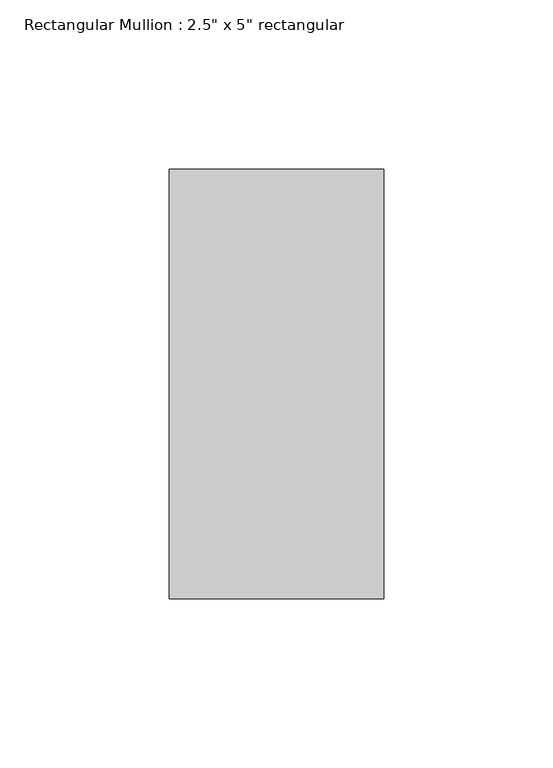
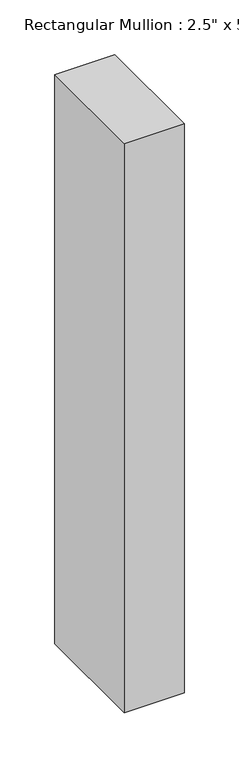
"""IFC4 building model written with IfcOpenShell, lengths in millimetres: member geometry."""

from ifc_helpers import new_model, si_unit, frame, origin, place, context, project, spatial, polyline, outline, extrude, source, transform, mapped, element, save


def member_057e2f1d(model_context):
    return source(origin(), model_context, "Body", "SweptSolid", [
        extrude(outline(polyline([(31.75, 63.5), (31.75, -63.5), (-31.75, -63.5), (-31.75, 63.5), (31.75, 63.5)])), frame((0.0, 0.0, -636.2206626), z_axis=(0.0, 0.0, 1.0), x_axis=(1.0, 0.0, 0.0)), (0.0, 0.0, 1.0), 636.2206626),
    ])


if __name__ == "__main__":
    model = new_model("IFC4")
    model_context = context("Model", 3, world=origin())
    ifc_project = project(units=[si_unit("LENGTHUNIT", "METRE", prefix="MILLI")], contexts=[model_context])
    site = spatial("IfcSite", under=ifc_project)
    building = spatial("IfcBuilding", under=site)
    placement = place(None, origin())
    member_shape = member_057e2f1d(model_context)
    element("IfcMember", 1, ObjectType="Rectangular Mullion : 2.5\" x 5\" rectangular", at=placement, inside=building, context=model_context, shape_type="MappedRepresentation", body=[
        mapped(member_shape, transform((0.0, 0.0, 0.0), x_axis=(1.0, 0.0, 0.0), y_axis=(0.0, 1.0, 0.0), z_axis=(0.0, 0.0, 1.0))),
    ])
    save(model, "model.ifc")

# Revit data of these elements
# Type "Rectangular Mullion : 2.5\" x 5\" rectangular"
#   built-in parameter 1007304 = 0.416667 (stored number, unit not read)
#   built-in parameter 1007301 = 0.104167 (stored number, unit not read)
#   built-in parameter 1007300 = 0.104167 (stored number, unit not read)
# Element 1 (IfcMember, "Rectangular Mullion : 2.5\" x 5\" rectangular")
#   Materials on its faces: "Aluminum"
# Materials
#   "Aluminum": class "Metal", colour RGB 247 247 247, transparency 0, Description = "Aluminum 6061", Cost = 0
